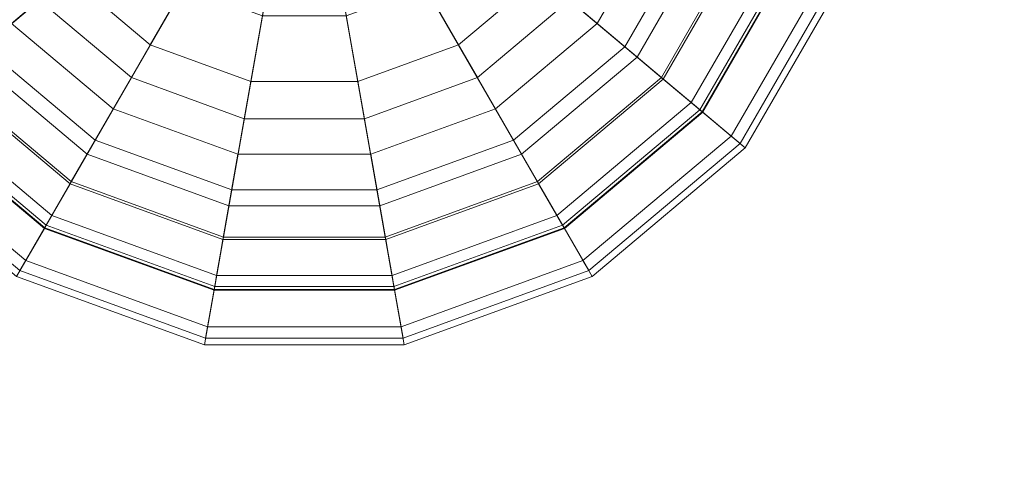
# Model space of a CAD drawing. Units: inches. Extents: x 375 to 1122, y 27 to 1069.
# Tile 98 of 155: x 718.593 to 720.91, y 863.668 to 864.699. Entities that reach past the tile are written whole.
import ezdxf

# ---------------------------------------------------------------- set-up
doc = ezdxf.new("R2010")
doc.units = ezdxf.units.IN
doc.layers.add('A-ANNO-DIMS', color=2, linetype='Continuous', lineweight=18)
doc.layers.add('Furniture', color=30, linetype='Continuous', lineweight=18)
doc.styles.get("Standard").update_dxf_attribs({"font": 'arial.ttf'})
doc.dimstyles.new('ISO-25', dxfattribs={"dimtxt": 12, "dimasz": 2.5, "dimexe": 1.5, "dimexo": 1.5, "dimtad": 1, "dimdec": 1, "dimlunit": 3, "dimtxsty": 'Standard', "dimblk": 'ARCHTICK', "dimcen": 2.5, "dimadec": 0, "dimazin": 0, "dimtfac": 1, "dimtdec": 1, "dimtmove": 0, "dimatfit": 3, "dimfxl": 1.5, "dimfxlon": 1, "dimarcsym": 0})

# ---------------------------------------------------------------- blocks, each defined once
blk = doc.blocks.new('A$C403C54AD')
for points in [[(1.848325, 0.883824, -0.031825), (1.826559, 0.857884, -0.028747), (1.826559, 0.857884, -0.028747), (1.83814, 0.889704, -0.031825)], [(1.8462, 0.881291, 0.131159), (1.848069, 0.883518, 0.117935), (1.838004, 0.889329, 0.117935), (1.83701, 0.886597, 0.131159)], [(1.846226, 0.881322, -0.028594), (1.848325, 0.883824, -0.031825), (1.83814, 0.889704, -0.031825), (1.837023, 0.886635, -0.028594)], [(1.848069, 0.883518, 0.117935), (1.847635, 0.883001, 0.089693), (1.837773, 0.888695, 0.089693), (1.838004, 0.889329, 0.117935)], [(1.847635, 0.883001, 0.089693), (1.844187, 0.878892, 0.071684), (1.835938, 0.883654, 0.071684), (1.837773, 0.888695, 0.089693)], [(1.835696, 0.868773, -0.02532), (1.846226, 0.881322, -0.028594), (1.837023, 0.886635, -0.028594), (1.83142, 0.871241, -0.02532)], [(1.842988, 0.877464, 0.140564), (1.8462, 0.881291, 0.131159), (1.83701, 0.886597, 0.131159), (1.835301, 0.881902, 0.140564)], [(1.846086, 0.881156, 0.117718), (1.84428, 0.879003, 0.130354), (1.835988, 0.88379, 0.130354), (1.836949, 0.886431, 0.117718)], [(1.845663, 0.880651, 0.090178), (1.846086, 0.881156, 0.117718), (1.836949, 0.886431, 0.117718), (1.836724, 0.885812, 0.090178)], [(1.84238, 0.876739, 0.073031), (1.845663, 0.880651, 0.090178), (1.836724, 0.885812, 0.090178), (1.834977, 0.881013, 0.073031)], [(1.855884, 0.874815, -0.031825), (1.826559, 0.857884, -0.028747), (1.826559, 0.857884, -0.028747), (1.848325, 0.883824, -0.031825)], [(1.844187, 0.878892, 0.071684), (1.839644, 0.873479, 0.061451), (1.833522, 0.877014, 0.061451), (1.835938, 0.883654, 0.071684)], [(1.84428, 0.879003, 0.130354), (1.84101, 0.875106, 0.140564), (1.834248, 0.879009, 0.140564), (1.835988, 0.88379, 0.130354)], [(1.853021, 0.873162, 0.131159), (1.855539, 0.874616, 0.117935), (1.848069, 0.883518, 0.117935), (1.8462, 0.881291, 0.131159)], [(1.853056, 0.873182, -0.028594), (1.855884, 0.874815, -0.031825), (1.848325, 0.883824, -0.031825), (1.846226, 0.881322, -0.028594)], [(1.855539, 0.874616, 0.117935), (1.854954, 0.874278, 0.089693), (1.847635, 0.883001, 0.089693), (1.848069, 0.883518, 0.117935)], [(1.854954, 0.874278, 0.089693), (1.850309, 0.871596, 0.071684), (1.844187, 0.878892, 0.071684), (1.847635, 0.883001, 0.089693)], [(1.84101, 0.875106, 0.140564), (1.842988, 0.877464, 0.140564), (1.835301, 0.881902, 0.140564), (1.834248, 0.879009, 0.140564)], [(1.838869, 0.864991, -0.02532), (1.853056, 0.873182, -0.028594), (1.846226, 0.881322, -0.028594), (1.835696, 0.868773, -0.02532)], [(1.848694, 0.870664, 0.140564), (1.853021, 0.873162, 0.131159), (1.8462, 0.881291, 0.131159), (1.842988, 0.877464, 0.140564)], [(1.852868, 0.873073, 0.117718), (1.850434, 0.871669, 0.130354), (1.84428, 0.879003, 0.130354), (1.846086, 0.881156, 0.117718)], [(1.852298, 0.872744, 0.090178), (1.852868, 0.873073, 0.117718), (1.846086, 0.881156, 0.117718), (1.845663, 0.880651, 0.090178)], [(1.838211, 0.87177, 0.063639), (1.84238, 0.876739, 0.073031), (1.834977, 0.881013, 0.073031), (1.832759, 0.874918, 0.063639)], [(1.847874, 0.87019, 0.073031), (1.852298, 0.872744, 0.090178), (1.845663, 0.880651, 0.090178), (1.84238, 0.876739, 0.073031)], [(1.850309, 0.871596, 0.071684), (1.844189, 0.868063, 0.061451), (1.839644, 0.873479, 0.061451), (1.844187, 0.878892, 0.071684)], [(1.850434, 0.871669, 0.130354), (1.846028, 0.869125, 0.140564), (1.84101, 0.875106, 0.140564), (1.84428, 0.879003, 0.130354)], [(1.846028, 0.869125, 0.140564), (1.848694, 0.870664, 0.140564), (1.842988, 0.877464, 0.140564), (1.84101, 0.875106, 0.140564)], [(1.842258, 0.866948, 0.063639), (1.847874, 0.87019, 0.073031), (1.84238, 0.876739, 0.073031), (1.838211, 0.87177, 0.063639)], [(1.859907, 0.863764, -0.031825), (1.826559, 0.857884, -0.028747), (1.826559, 0.857884, -0.028747), (1.855884, 0.874815, -0.031825)], [(1.85669, 0.863197, -0.028594), (1.859907, 0.863764, -0.031825), (1.855884, 0.874815, -0.031825), (1.853056, 0.873182, -0.028594)], [(1.858849, 0.863578, 0.089693), (1.853566, 0.862646, 0.071684), (1.850309, 0.871596, 0.071684), (1.854954, 0.874278, 0.089693)], [(1.856651, 0.86319, 0.131159), (1.859514, 0.863695, 0.117935), (1.855539, 0.874616, 0.117935), (1.853021, 0.873162, 0.131159)], [(1.859514, 0.863695, 0.117935), (1.858849, 0.863578, 0.089693), (1.854954, 0.874278, 0.089693), (1.855539, 0.874616, 0.117935)], [(1.844189, 0.868063, 0.061451), (1.835322, 0.862943, 0.054084), (1.833063, 0.865635, 0.054084), (1.839644, 0.873479, 0.061451)], [(1.840557, 0.860352, -0.02532), (1.85669, 0.863197, -0.028594), (1.853056, 0.873182, -0.028594), (1.838869, 0.864991, -0.02532)], [(1.85173, 0.862322, 0.140564), (1.856651, 0.86319, 0.131159), (1.853021, 0.873162, 0.131159), (1.848694, 0.870664, 0.140564)], [(1.856476, 0.863159, 0.117718), (1.853709, 0.862671, 0.130354), (1.850434, 0.871669, 0.130354), (1.852868, 0.873073, 0.117718)], [(1.855828, 0.863045, 0.090178), (1.856476, 0.863159, 0.117718), (1.852868, 0.873073, 0.117718), (1.852298, 0.872744, 0.090178)], [(1.850798, 0.862158, 0.073031), (1.855828, 0.863045, 0.090178), (1.852298, 0.872744, 0.090178), (1.847874, 0.87019, 0.073031)], [(1.83427, 0.862336, 0.057003), (1.842258, 0.866948, 0.063639), (1.838211, 0.87177, 0.063639), (1.832282, 0.864705, 0.057003)], [(1.853566, 0.862646, 0.071684), (1.846607, 0.861419, 0.061451), (1.844189, 0.868063, 0.061451), (1.850309, 0.871596, 0.071684)], [(1.853709, 0.862671, 0.130354), (1.848699, 0.861788, 0.140564), (1.846028, 0.869125, 0.140564), (1.850434, 0.871669, 0.130354)], [(1.844411, 0.861032, 0.063639), (1.850798, 0.862158, 0.073031), (1.847874, 0.87019, 0.073031), (1.842258, 0.866948, 0.063639)], [(1.848699, 0.861788, 0.140564), (1.85173, 0.862322, 0.140564), (1.848694, 0.870664, 0.140564), (1.846028, 0.869125, 0.140564)], [(1.846607, 0.861419, 0.061451), (1.836524, 0.859641, 0.054084), (1.835322, 0.862943, 0.054084), (1.844189, 0.868063, 0.061451)], [(1.835328, 0.85943, 0.057003), (1.844411, 0.861032, 0.063639), (1.842258, 0.866948, 0.063639), (1.83427, 0.862336, 0.057003)], [(1.859907, 0.852004, -0.031825), (1.826559, 0.857884, -0.028747), (1.826559, 0.857884, -0.028747), (1.859907, 0.863764, -0.031825)], [(1.840557, 0.855416, -0.02532), (1.85669, 0.852571, -0.028594), (1.85669, 0.863197, -0.028594), (1.840557, 0.860352, -0.02532)], [(1.858849, 0.85219, 0.089693), (1.853566, 0.853122, 0.071684), (1.853566, 0.862646, 0.071684), (1.858849, 0.863578, 0.089693)], [(1.856651, 0.852578, 0.131159), (1.859514, 0.852073, 0.117935), (1.859514, 0.863695, 0.117935), (1.856651, 0.86319, 0.131159)], [(1.85669, 0.852571, -0.028594), (1.859907, 0.852004, -0.031825), (1.859907, 0.863764, -0.031825), (1.85669, 0.863197, -0.028594)], [(1.859514, 0.852073, 0.117935), (1.858849, 0.85219, 0.089693), (1.858849, 0.863578, 0.089693), (1.859514, 0.863695, 0.117935)], [(1.853566, 0.853122, 0.071684), (1.846607, 0.854349, 0.061451), (1.846607, 0.861419, 0.061451), (1.853566, 0.862646, 0.071684)], [(1.853709, 0.853097, 0.130354), (1.848699, 0.85398, 0.140564), (1.848699, 0.861788, 0.140564), (1.853709, 0.862671, 0.130354)], [(1.850798, 0.85361, 0.073031), (1.855828, 0.852723, 0.090178), (1.855828, 0.863045, 0.090178), (1.850798, 0.862158, 0.073031)], [(1.85173, 0.853446, 0.140564), (1.856651, 0.852578, 0.131159), (1.856651, 0.86319, 0.131159), (1.85173, 0.862322, 0.140564)], [(1.856476, 0.852609, 0.117718), (1.853709, 0.853097, 0.130354), (1.853709, 0.862671, 0.130354), (1.856476, 0.863159, 0.117718)], [(1.855828, 0.852723, 0.090178), (1.856476, 0.852609, 0.117718), (1.856476, 0.863159, 0.117718), (1.855828, 0.863045, 0.090178)], [(1.844411, 0.854736, 0.063639), (1.850798, 0.85361, 0.073031), (1.850798, 0.862158, 0.073031), (1.844411, 0.861032, 0.063639)], [(1.848699, 0.85398, 0.140564), (1.85173, 0.853446, 0.140564), (1.85173, 0.862322, 0.140564), (1.848699, 0.861788, 0.140564)], [(1.835328, 0.856338, 0.057003), (1.844411, 0.854736, 0.063639), (1.844411, 0.861032, 0.063639), (1.835328, 0.85943, 0.057003)], [(1.846607, 0.854349, 0.061451), (1.836524, 0.856127, 0.054084), (1.836524, 0.859641, 0.054084), (1.846607, 0.861419, 0.061451)], [(1.855884, 0.840953, -0.031825), (1.826559, 0.857884, -0.028747), (1.826559, 0.857884, -0.028747), (1.859907, 0.852004, -0.031825)], [(1.848325, 0.831944, -0.031825), (1.826559, 0.857884, -0.028747), (1.826559, 0.857884, -0.028747), (1.855884, 0.840953, -0.031825)], [(1.83814, 0.826064, -0.031825), (1.826559, 0.857884, -0.028747), (1.826559, 0.857884, -0.028747), (1.848325, 0.831944, -0.031825)], [(1.83427, 0.853432, 0.057003), (1.842258, 0.84882, 0.063639), (1.844411, 0.854736, 0.063639), (1.835328, 0.856338, 0.057003)], [(1.844189, 0.847705, 0.061451), (1.835322, 0.852825, 0.054084), (1.836524, 0.856127, 0.054084), (1.846607, 0.854349, 0.061451)], [(1.838869, 0.850777, -0.02532), (1.853056, 0.842586, -0.028594), (1.85669, 0.852571, -0.028594), (1.840557, 0.855416, -0.02532)], [(1.842258, 0.84882, 0.063639), (1.847874, 0.845577, 0.073031), (1.850798, 0.85361, 0.073031), (1.844411, 0.854736, 0.063639)], [(1.850309, 0.844172, 0.071684), (1.844189, 0.847705, 0.061451), (1.846607, 0.854349, 0.061451), (1.853566, 0.853122, 0.071684)], [(1.846028, 0.846643, 0.140564), (1.848694, 0.845104, 0.140564), (1.85173, 0.853446, 0.140564), (1.848699, 0.85398, 0.140564)], [(1.850434, 0.844099, 0.130354), (1.846028, 0.846643, 0.140564), (1.848699, 0.85398, 0.140564), (1.853709, 0.853097, 0.130354)], [(1.832282, 0.851063, 0.057003), (1.838211, 0.843998, 0.063639), (1.842258, 0.84882, 0.063639), (1.83427, 0.853432, 0.057003)], [(1.847874, 0.845577, 0.073031), (1.852298, 0.843024, 0.090178), (1.855828, 0.852723, 0.090178), (1.850798, 0.85361, 0.073031)], [(1.848694, 0.845104, 0.140564), (1.853021, 0.842606, 0.131159), (1.856651, 0.852578, 0.131159), (1.85173, 0.853446, 0.140564)], [(1.839644, 0.842289, 0.061451), (1.833063, 0.850133, 0.054084), (1.835322, 0.852825, 0.054084), (1.844189, 0.847705, 0.061451)], [(1.854954, 0.84149, 0.089693), (1.850309, 0.844172, 0.071684), (1.853566, 0.853122, 0.071684), (1.858849, 0.85219, 0.089693)], [(1.852868, 0.842695, 0.117718), (1.850434, 0.844099, 0.130354), (1.853709, 0.853097, 0.130354), (1.856476, 0.852609, 0.117718)], [(1.852298, 0.843024, 0.090178), (1.852868, 0.842695, 0.117718), (1.856476, 0.852609, 0.117718), (1.855828, 0.852723, 0.090178)], [(1.853021, 0.842606, 0.131159), (1.855539, 0.841152, 0.117935), (1.859514, 0.852073, 0.117935), (1.856651, 0.852578, 0.131159)], [(1.853056, 0.842586, -0.028594), (1.855884, 0.840953, -0.031825), (1.859907, 0.852004, -0.031825), (1.85669, 0.852571, -0.028594)], [(1.855539, 0.841152, 0.117935), (1.854954, 0.84149, 0.089693), (1.858849, 0.85219, 0.089693), (1.859514, 0.852073, 0.117935)], [(1.835696, 0.846995, -0.02532), (1.846226, 0.834446, -0.028594), (1.853056, 0.842586, -0.028594), (1.838869, 0.850777, -0.02532)], [(1.838211, 0.843998, 0.063639), (1.84238, 0.839029, 0.073031), (1.847874, 0.845577, 0.073031), (1.842258, 0.84882, 0.063639)], [(1.844187, 0.836876, 0.071684), (1.839644, 0.842289, 0.061451), (1.844189, 0.847705, 0.061451), (1.850309, 0.844172, 0.071684)], [(1.83142, 0.844527, -0.02532), (1.837023, 0.829133, -0.028594), (1.846226, 0.834446, -0.028594), (1.835696, 0.846995, -0.02532)], [(1.84101, 0.840662, 0.140564), (1.842988, 0.838304, 0.140564), (1.848694, 0.845104, 0.140564), (1.846028, 0.846643, 0.140564)], [(1.84428, 0.836765, 0.130354), (1.84101, 0.840662, 0.140564), (1.846028, 0.846643, 0.140564), (1.850434, 0.844099, 0.130354)], [(1.84238, 0.839029, 0.073031), (1.845663, 0.835117, 0.090178), (1.852298, 0.843024, 0.090178), (1.847874, 0.845577, 0.073031)], [(1.842988, 0.838304, 0.140564), (1.8462, 0.834477, 0.131159), (1.853021, 0.842606, 0.131159), (1.848694, 0.845104, 0.140564)], [(1.847635, 0.832767, 0.089693), (1.844187, 0.836876, 0.071684), (1.850309, 0.844172, 0.071684), (1.854954, 0.84149, 0.089693)], [(1.846086, 0.834612, 0.117718), (1.84428, 0.836765, 0.130354), (1.850434, 0.844099, 0.130354), (1.852868, 0.842695, 0.117718)], [(1.832759, 0.84085, 0.063639), (1.834977, 0.834755, 0.073031), (1.84238, 0.839029, 0.073031), (1.838211, 0.843998, 0.063639)], [(1.845663, 0.835117, 0.090178), (1.846086, 0.834612, 0.117718), (1.852868, 0.842695, 0.117718), (1.852298, 0.843024, 0.090178)], [(1.8462, 0.834477, 0.131159), (1.848069, 0.83225, 0.117935), (1.855539, 0.841152, 0.117935), (1.853021, 0.842606, 0.131159)], [(1.846226, 0.834446, -0.028594), (1.848325, 0.831944, -0.031825), (1.855884, 0.840953, -0.031825), (1.853056, 0.842586, -0.028594)], [(1.835938, 0.832114, 0.071684), (1.833522, 0.838754, 0.061451), (1.839644, 0.842289, 0.061451), (1.844187, 0.836876, 0.071684)], [(1.848069, 0.83225, 0.117935), (1.847635, 0.832767, 0.089693), (1.854954, 0.84149, 0.089693), (1.855539, 0.841152, 0.117935)]]:
    blk.add_3dface(points)
blk = doc.blocks.new('_ArchTick')
at = {"color": 0, "linetype": 'ByBlock', "const_width": 0.15}
blk.add_lwpolyline([(-0.5, -0.5), (0.5, 0.5)], dxfattribs=at)
blk = doc.blocks.new('*D85')
at = {"layer": 'A-ANNO-DIMS', "color": 0, "lineweight": -2, "transparency": 16777216}
for p, q in [((401.5073, 868.5277), (398.5073, 868.5277)), ((400.0073, 814.5277), (400.0073, 868.5277)), ((401.5073, 814.5277), (398.5073, 814.5277))]:
    blk.add_line(p, q, dxfattribs=at)
at = {"layer": 'Defpoints', "color": 0, "transparency": 16777216}
for p in [(400.0073, 868.5277), (845.0073, 868.5277), (845.0073, 814.5277)]:
    blk.add_point(p, dxfattribs=at)
at = {"layer": 'A-ANNO-DIMS', "color": 0, "lineweight": -2, "transparency": 16777216, "xscale": 2.5, "yscale": 2.5, "zscale": 2.5}
for p, rotation in [((400.0073, 868.5277), 90), ((400.0073, 814.5277), 270)]:
    blk.add_blockref('_ArchTick', p, dxfattribs=dict(at, rotation=rotation))
at = {"layer": 'A-ANNO-DIMS', "color": 0, "transparency": 16777216, "insert": (393.2555, 841.5277), "char_height": 12, "attachment_point": 5, "rotation": 90}
blk.add_mtext('4\'-6"', dxfattribs=at)

msp = doc.modelspace()

# ---------------------------------------------------------------- block references
at = {"layer": 'Furniture', "xscale": 39.9918517141215, "yscale": 39.9918517141215, "zscale": 39.9918517141215, "rotation": 270}
msp.add_blockref('A$C403C54AD', (684.9549, 938.3156, 0.024), dxfattribs=at)

# ---------------------------------------------------------------- dimensions: what is measured, and where the dimension line sits
at = {"layer": 'A-ANNO-DIMS'}
dim = msp.add_linear_dim(base=(400.0073, 868.5277), p1=(845.0073, 814.5277), p2=(845.0073, 868.5277), angle=90, dimstyle='ISO-25', override={"dimdec": 1, "dimlfac": 1, "dimrnd": 0, "dimzin": 1, "dimdsep": 46, "dimlunit": 4, "dimfrac": 2}, dxfattribs=at)
dim.commit()
dim.dimension.update_dxf_attribs({"geometry": '*D85', "text_midpoint": (393.2555, 841.5277)})

doc.saveas('drawing.dxf')
